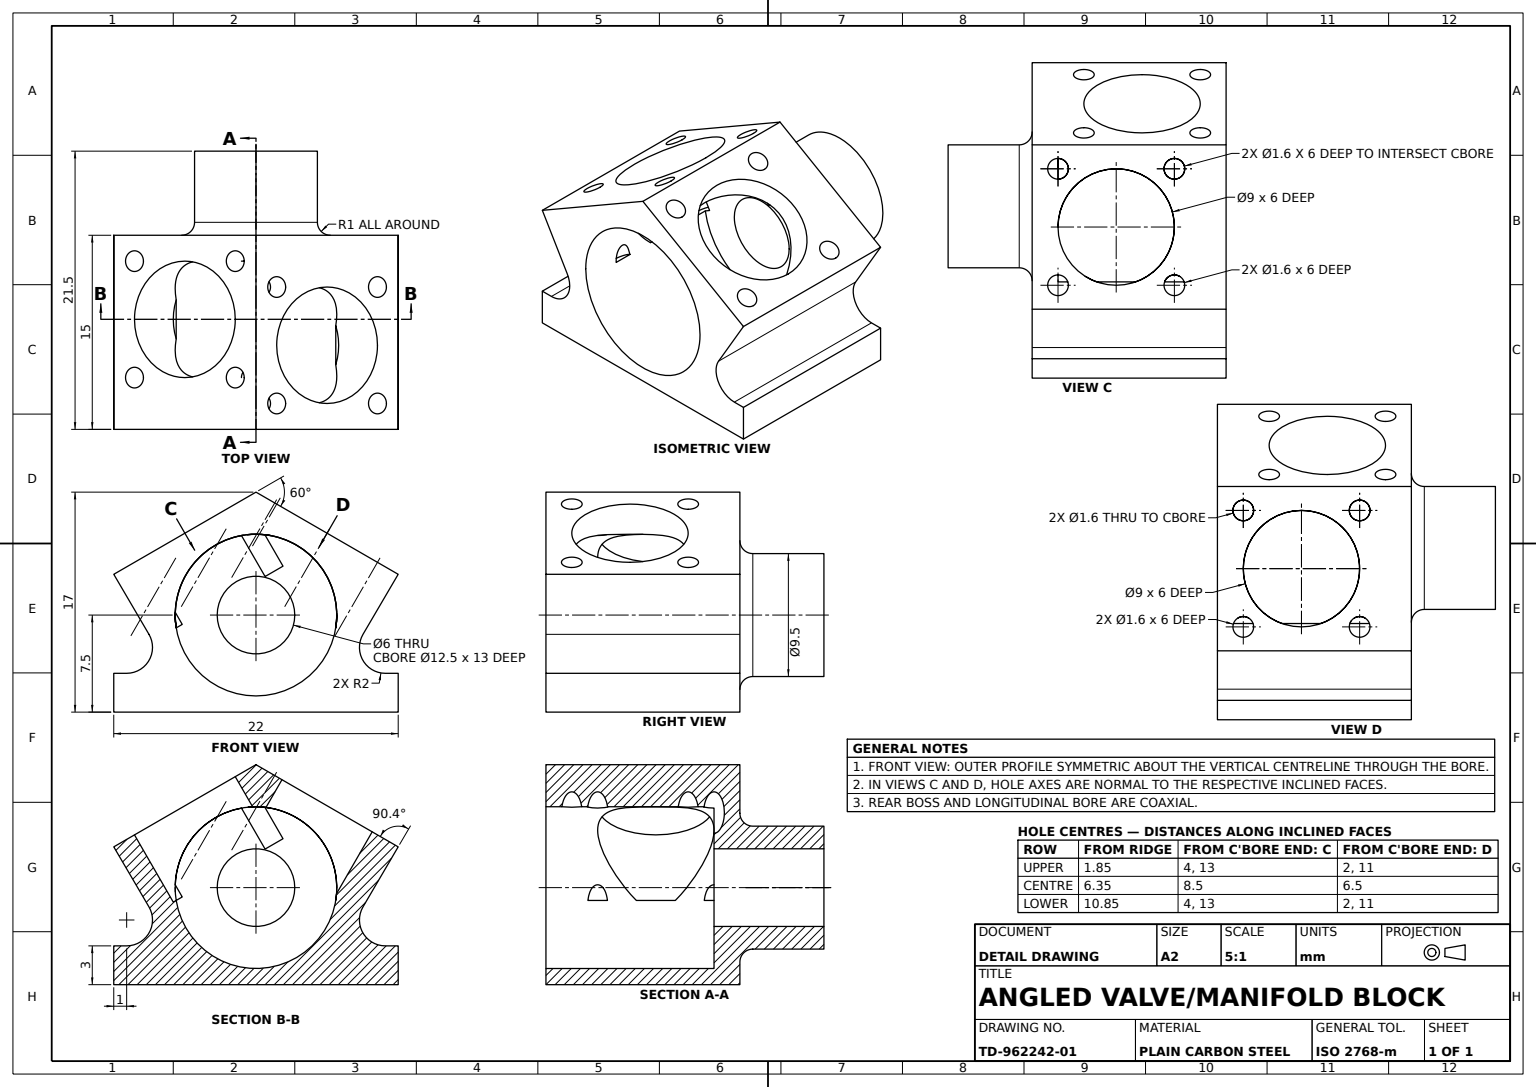
SolidWorks part; units mm, degrees
material "Plain Carbon Steel"
ref_plane "Front Plane" through (0, 0, 0) normal (0, 0, 1) x (1, 0, 0)
ref_plane "Top Plane" through (0, 0, 0) normal (0, 1, 0) x (1, 0, 0)
ref_plane "Right Plane" through (0, 0, 0) normal (1, 0, 0) x (0, 0, -1)
sketch "Housing Profile Sketch" plane through (0, 0, 0) normal (0, 0, 1) x (1, 0, 0)
  line L1 (0, 17) -> (-10.9985, 10.65)
  line L2 (0, 17) -> (10.9985, 10.65)
  line L3 (-10.0021, 0) -> (10.0021, 0)
  line L4 (-10.0021, 0) -> (-11, 0)
  line L5 (10.0021, 0) -> (11, 0)
  line L6 (11, 0) -> (11, 2.9988)
  line L7 (11, 2.9988) -> (10.0021, 2.9988)
  line L8 (10.9985, 10.65) -> (8.277, 6.0107)
  line L9 (-11, 2.9988) -> (-10.0021, 2.9988)
  line L10 (-11, 0) -> (-11, 2.9988)
  line L11 (-10.9985, 10.65) -> (-8.277, 6.0107)
  arc A0 (8.277, 6.0107) -> (10.0021, 2.9988) centre (10.0021, 4.9988) ccw
  arc A1 (-8.277, 6.0107) -> (-10.0021, 2.9988) centre (-10.0021, 4.9988) cw
  circle A2 centre (0, 7.5) radius 6.25
  dimension "D1" = 11
  dimension "D5" = 2
  dimension "D10" = 12.5
  dimension "D2" = 11
  dimension "D3" = 2.9988
  dimension "D4" = 0.9979
  dimension "D6" = 17
  dimension "D7" = 10.65
  dimension "D8" = 12.7
  dimension "D9" = 7.5
extrude "Housing Body" add sketch "Housing Profile Sketch" against normal blind 15
sketch "Cylindrical Boss Sketch" plane through (0, 0, -15) normal (0, 0, -1) x (-1, 0, 0)
  line L0 (-11, 0) -> (-11, 2.9988) construction
  line L1 (-11, 2.9988) -> (-10.0021, 2.9988) construction
  circle A0 centre (0, 7.5) radius 4.75
  dimension "D1" = 9.5
  dimension "D2" = 11
  dimension "D3" = 4.5012
extrude "Cylindrical Boss" add sketch "Cylindrical Boss Sketch" along normal blind 6.5 separate body
sketch "Boss Collar Sketch" plane through (0, 0, -15) normal (0, 0, -1) x (-1, 0, 0)
  circle A0 centre (0, 7.5) radius 6.25
  dimension "D1" = 12.5
extrude "Boss Collar" add sketch "Boss Collar Sketch" against normal blind 2
sketch "Through Bore Sketch" plane through (0, 0, -21.5) normal (0, 0, -1) x (-1, 0, 0)
  circle A0 centre (0, 7.5) radius 3
  dimension "D1" = 6
extrude "Through Bore" cut sketch "Through Bore Sketch" against normal blind 43
sketch "Face Holes A Sketch" plane through (7.3612, 12.75, 0) normal (0.5, 0.866, 0) x (0.866, -0.5, 0)
  line L0 (4.2, 15) -> (4.2, 0) construction
  circle A0 centre (-2.15, 6.5) radius 4.5
  circle A1 centre (2.35, 11) radius 0.8
  circle A2 centre (2.35, 2) radius 0.8
  circle A3 centre (-6.65, 2) radius 0.8
  circle A4 centre (-6.65, 11) radius 0.8
  dimension "D1" = 6.5
  dimension "D6" = 9
  dimension "D7" = 1.6
  dimension "D2" = 2
  dimension "D3" = 2
  dimension "D4" = 11
  dimension "D5" = 11
  dimension "D8" = 1.85
  dimension "D9" = 6.35
  dimension "D10" = 10.85
extrude "Face Holes A" cut sketch "Face Holes A Sketch" against normal blind 6
sketch "Face Holes B Sketch" plane through (-7.3612, 12.75, 0) normal (-0.5, 0.866, 0) x (0.866, 0.5, 0)
  circle A0 centre (2.15, 8.5) radius 4.5
  circle A1 centre (-2.35, 13) radius 0.8
  circle A2 centre (6.65, 13) radius 0.8
  circle A3 centre (6.65, 4) radius 0.8
  circle A4 centre (-2.35, 4) radius 0.8
  dimension "D1" = 1.6
  dimension "D2" = 1.6
  dimension "D3" = 1.6
  dimension "D4" = 1.6
  dimension "D5" = 9
  dimension "D6" = 8.5
  dimension "D7" = 13
  dimension "D8" = 2.35
  dimension "D9" = 2.15
  dimension "D10" = 4
  dimension "D11" = 2.35
  dimension "D12" = 6.65
  dimension "D13" = 4
  dimension "D14" = 4.5
  dimension "D15" = 4.5
extrude "Face Holes B" cut sketch "Face Holes B Sketch" against normal blind 6
fillet "Edge Fillet R1" radius 1 1 edges at (-4.75, 7.5, -15)
